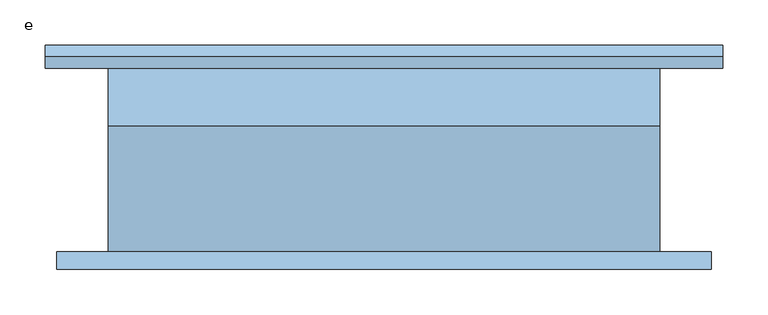
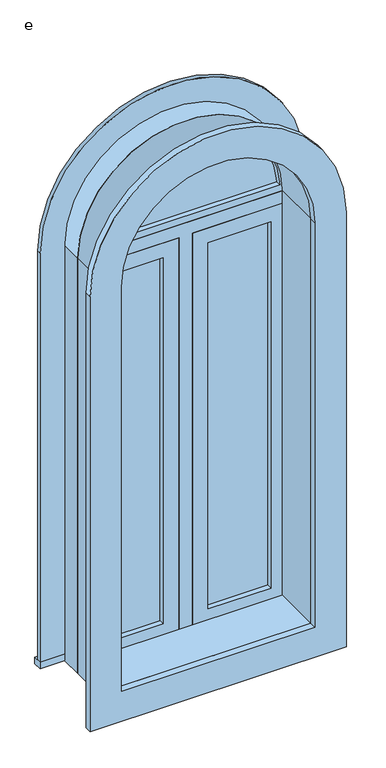
"""IFC4 building model written with IfcOpenShell, lengths in millimetres: window geometry, e."""

from ifc_helpers import new_model, si_unit, point, frame, frame_2d, origin, place, context, project, spatial, polyline, circle_curve, trimmed, segment, composite_curve, outline, extrude, source, transform, mapped, element, save


def e_49ac7ee0(model_context):
    return source(origin(), model_context, "Body", "SweptSolid", [
        extrude(outline(composite_curve([segment(polyline([(1543.05, -353.9478419), (247.65, -353.9478419), (247.65, 369.9521581), (1543.05, 369.9521581)]), True, "CONTINUOUS"), segment(trimmed(circle_curve(frame_2d((1543.05, 8.0021581)), 361.95), [point((1543.05, 369.9521581))], [point((1543.05, -353.9478419))], False, "CARTESIAN"), True, "CONTINUOUS")], self_intersect=False), holes=[composite_curve([segment(trimmed(circle_curve(frame_2d((1543.05, 8.0021581)), 273.05), [point((1543.05, -265.0478419))], [point((1543.05, 281.0521581))], True, "CARTESIAN"), True, "CONTINUOUS"), segment(polyline([(1543.05, 281.0521581), (336.55, 281.0521581), (336.55, -265.0478419), (1543.05, -265.0478419)]), True, "CONTINUOUS")], self_intersect=False)]), frame((0.0, -120.65, 0.0), z_axis=(0.0, 1.0, 0.0), x_axis=(0.0, 0.0, 1.0)), (0.0, 0.0, 1.0), 19.05),
        extrude(outline(composite_curve([segment(trimmed(circle_curve(frame_2d((1543.05, 8.0021581)), 267.0627113), [point((1562.0999995, 274.3845699))], [point((1562.0999995, -258.3802537))], False, "CARTESIAN"), True, "CONTINUOUS"), segment(polyline([(1562.0999995, -258.3802537), (1562.0999995, 274.3845699)]), True, "CONTINUOUS")], self_intersect=False)), frame((0.0, 53.975, 0.0), z_axis=(0.0, 1.0, 0.0), x_axis=(0.0, 0.0, 1.0)), (0.0, 0.0, 1.0), 12.7),
        extrude(outline(composite_curve([segment(trimmed(circle_curve(frame_2d((1543.05, 8.0021581)), 285.75), [point((1543.05, 293.7521581))], [point((1543.05, -277.7478419))], False, "CARTESIAN"), True, "CONTINUOUS"), segment(polyline([(1543.05, -277.7478419), (1543.05, 293.7521581)]), True, "CONTINUOUS")], self_intersect=False), holes=[composite_curve([segment(polyline([(1562.0999995, 274.3845698), (1562.0999995, -258.3802537)]), True, "CONTINUOUS"), segment(trimmed(circle_curve(frame_2d((1543.05, 8.0021581)), 267.0627113), [point((1562.0999995, -258.3802537))], [point((1562.0999995, 274.3845698))], True, "CARTESIAN"), True, "CONTINUOUS")], self_intersect=False)]), frame((0.0, 38.1, 0.0), z_axis=(0.0, 1.0, 0.0), x_axis=(0.0, 0.0, 1.0)), (0.0, 0.0, 1.0), 44.45),
        extrude(outline(composite_curve([segment(polyline([(304.8, -296.7978419), (304.8, 312.8021581), (1543.05, 312.8021581)]), True, "CONTINUOUS"), segment(trimmed(circle_curve(frame_2d((1543.05, 8.0021581)), 304.8), [point((1543.05, 312.8021581))], [point((1543.05, -296.7978419))], False, "CARTESIAN"), True, "CONTINUOUS"), segment(polyline([(1543.05, -296.7978419), (304.8, -296.7978419)]), True, "CONTINUOUS")], self_intersect=False), holes=[composite_curve([segment(polyline([(323.85, -277.7478419), (1543.05, -277.7478419)]), True, "CONTINUOUS"), segment(trimmed(circle_curve(frame_2d((1543.05, 8.0021581)), 285.75), [point((1543.05, -277.7478419))], [point((1543.05, 293.7521581))], True, "CARTESIAN"), True, "CONTINUOUS"), segment(polyline([(1543.05, 293.7521581), (323.85, 293.7521581), (323.85, -277.7478419)]), True, "CONTINUOUS")], self_intersect=False)]), frame((0.0, 38.1, 0.0), z_axis=(0.0, 1.0, 0.0), x_axis=(0.0, 0.0, 1.0)), (0.0, 0.0, 1.0), 63.5),
        extrude(outline(polyline([(71.5021581, 66.675), (249.3021581, 66.675), (249.3021581, 53.975), (71.5021581, 53.975), (71.5021581, 66.675)])), frame((0.0, 0.0, 368.3), z_axis=(0.0, 0.0, 1.0), x_axis=(1.0, 0.0, 0.0)), (0.0, 0.0, 1.0), 1092.2),
        extrude(outline(polyline([(1504.95, 27.0521581), (323.85, 27.0521581), (323.85, 293.7521581), (1504.95, 293.7521581), (1504.95, 27.0521581)]), holes=[polyline([(1460.5, 71.5021581), (1460.5, 249.3021581), (368.3, 249.3021581), (368.3, 71.5021581), (1460.5, 71.5021581)])]), frame((0.0, 38.1, 0.0), z_axis=(0.0, 1.0, 0.0), x_axis=(0.0, 0.0, 1.0)), (0.0, 0.0, 1.0), 44.45),
        extrude(outline(polyline([(323.85, -11.0478419), (323.85, 27.0521581), (1504.95, 27.0521581), (1504.95, 293.7521581), (1543.05, 293.7521581), (1543.05, -277.7478419), (1504.95, -277.7478419), (1504.95, -11.0478419), (323.85, -11.0478419)])), frame((0.0, 38.1, 0.0), z_axis=(0.0, 1.0, 0.0), x_axis=(0.0, 0.0, 1.0)), (0.0, 0.0, 1.0), 63.5),
        extrude(outline(polyline([(-366.6478419, 127.0), (382.6521581, 127.0), (382.6521581, 101.6), (-366.6478419, 101.6), (-366.6478419, 127.0)])), frame((0.0, 0.0, 304.8), z_axis=(0.0, 0.0, 1.0), x_axis=(1.0, 0.0, 0.0)), (0.0, 0.0, 1.0), 19.05),
        extrude(outline(composite_curve([segment(polyline([(323.85, 293.7521581), (323.85, 382.6521581), (1543.05, 382.6521581)]), True, "CONTINUOUS"), segment(trimmed(circle_curve(frame_2d((1543.05, 8.0021581)), 374.65), [point((1543.05, 382.6521581))], [point((1543.05, -366.6478419))], False, "CARTESIAN"), True, "CONTINUOUS"), segment(polyline([(1543.05, -366.6478419), (323.85, -366.6478419), (323.85, -277.7478419), (1543.05, -277.7478419)]), True, "CONTINUOUS"), segment(trimmed(circle_curve(frame_2d((1543.05, 8.0021581)), 285.75), [point((1543.05, -277.7478419))], [point((1543.05, 293.7521581))], True, "CARTESIAN"), True, "CONTINUOUS"), segment(polyline([(1543.05, 293.7521581), (323.85, 293.7521581)]), True, "CONTINUOUS")], self_intersect=False)), frame((0.0, 101.6, 0.0), z_axis=(0.0, 1.0, 0.0), x_axis=(0.0, 0.0, 1.0)), (0.0, 0.0, 1.0), 12.7),
        extrude(outline(polyline([(-55.4978419, 53.975), (-233.2978419, 53.975), (-233.2978419, 66.675), (-55.4978419, 66.675), (-55.4978419, 53.975)])), frame((0.0, 0.0, 368.3), z_axis=(0.0, 0.0, 1.0), x_axis=(1.0, 0.0, 0.0)), (0.0, 0.0, 1.0), 1092.2),
        extrude(outline(polyline([(1504.95, -277.7478419), (323.85, -277.7478419), (323.85, -11.0478419), (1504.95, -11.0478419), (1504.95, -277.7478419)]), holes=[polyline([(1460.5, -233.2978419), (1460.5, -55.4978419), (368.3, -55.4978419), (368.3, -233.2978419), (1460.5, -233.2978419)])]), frame((0.0, 38.1, 0.0), z_axis=(0.0, 1.0, 0.0), x_axis=(0.0, 0.0, 1.0)), (0.0, 0.0, 1.0), 44.45),
        extrude(outline(composite_curve([segment(polyline([(304.8, 312.8021581), (1543.05, 312.8021581)]), True, "CONTINUOUS"), segment(trimmed(circle_curve(frame_2d((1543.05, 8.0021581)), 304.8), [point((1543.05, 312.8021581))], [point((1543.05, -296.7978419))], False, "CARTESIAN"), True, "CONTINUOUS"), segment(polyline([(1543.05, -296.7978419), (304.8, -296.7978419), (304.8, 312.8021581)]), True, "CONTINUOUS")], self_intersect=False), holes=[composite_curve([segment(polyline([(336.55, 281.0521581), (336.55, -265.0478419), (1543.05, -265.0478419)]), True, "CONTINUOUS"), segment(trimmed(circle_curve(frame_2d((1543.05, 8.0021581)), 273.05), [point((1543.05, -265.0478419))], [point((1543.05, 281.0521581))], True, "CARTESIAN"), True, "CONTINUOUS"), segment(polyline([(1543.05, 281.0521581), (336.55, 281.0521581)]), True, "CONTINUOUS")], self_intersect=False)]), frame((0.0, -101.6, 0.0), z_axis=(0.0, 1.0, 0.0), x_axis=(0.0, 0.0, 1.0)), (0.0, 0.0, 1.0), 139.7),
    ])


if __name__ == "__main__":
    model = new_model("IFC4")
    model_context = context("Model", 3, world=origin())
    ifc_project = project(units=[si_unit("LENGTHUNIT", "METRE", prefix="MILLI")], contexts=[model_context])
    site = spatial("IfcSite", under=ifc_project)
    building = spatial("IfcBuilding", under=site)
    placement = place(None, origin())
    e_shape = e_49ac7ee0(model_context)
    element("IfcWindow", 1, ObjectType="e", at=placement, inside=building, context=model_context, shape_type="MappedRepresentation", body=[
        mapped(e_shape, transform((0.0, 0.0, 0.0), x_axis=(1.0, 0.0, 0.0), y_axis=(0.0, 1.0, 0.0), z_axis=(0.0, 0.0, 1.0))),
    ])
    save(model, "model.ifc")

# Revit data of these elements
# Type "e"
#   Type Mark = "14"
#   Construction Type Id = "SGL"
#   Assembly Code = "B2020100"
#   Analytic Construction = "Large single-glazed windows"
#   Visual Light Transmittance = 0.9
#   Solar Heat Gain Coefficient = 0.86
#   Heat Transfer Coefficient (U) = 0.979472 BTU/(h·ft²·°F)
#   Height = 4' - 0"
#   Default Sill Height = 1' - 0"
#   Trim Projection - Ext. = 0' - 0 1/2"
#   Trim Projection - Int. = 0' - 0 3/4"
#   Trim Width - Exterior = 0' - 3 1/2"
#   Trim Width - Interior = 0' - 3 1/2"
#   Width = 2' - 0"
#   Window Inset = 0' - 0 3/4"
#   Define Thermal Properties by = 1
#   Glass Pane Material = Glass
#   Sash Material = Sash
#   Trim Exterior Material = Trim
#   Trim Interior Material = Trim
#   Wall Closure = (empty or 0)
# Element 1 (IfcWindow, "e")
#   Materials on its faces: "Sash", "Trim", "Glass"
# Materials
#   "Glass": class "Glass", colour RGB 0 128 192, transparency 0.75, Description = "Soda Lime Glass", Cost = 0
#   "Sash": class "Wood", colour RGB 224 178 126, transparency 0
#   "Trim": class "Wood", colour RGB 224 178 126, transparency 0
